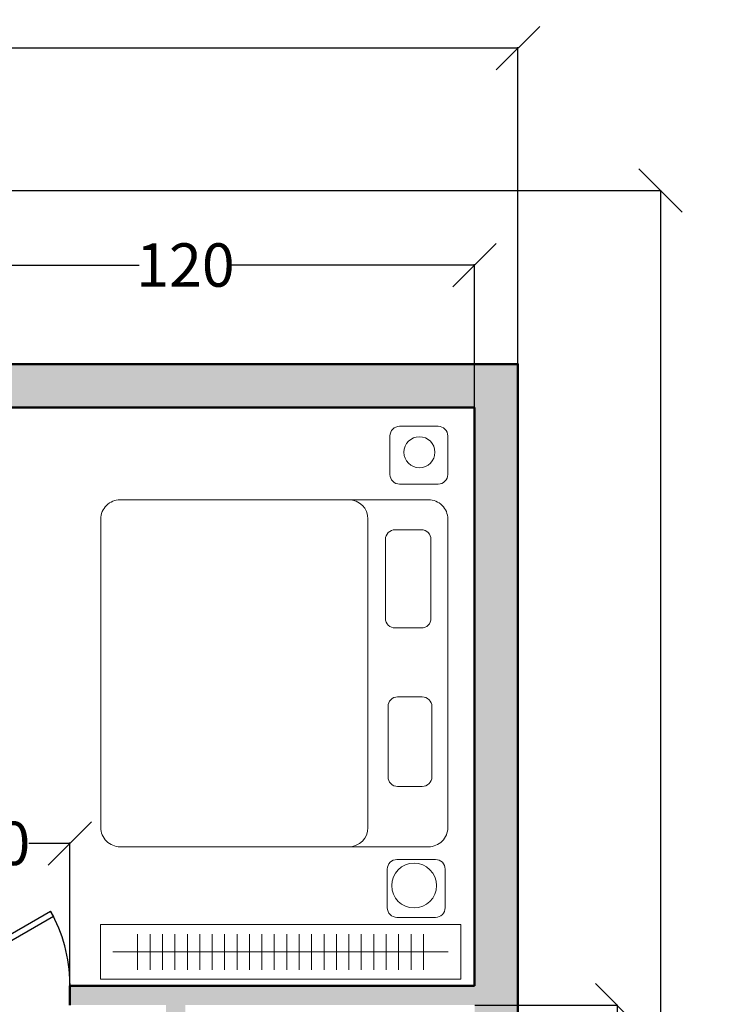
# Model space of a CAD drawing. Units: inches. Extents: x -9 to 615, y -420 to 89.
# Tile 6 of 6: x 467 to 615, y -115 to 89. Entities that reach past the tile are written whole.
import ezdxf

# ---------------------------------------------------------------- set-up
doc = ezdxf.new("R2010")
doc.units = ezdxf.units.IN
doc.header["$MEASUREMENT"] = 0
for name, color, linetype, lineweight in [('A-ANNO-DIMS', 2, 'Continuous', 18), ('A-DOOR', 4, 'Continuous', 25), ('A-FLOR-CASE', 32, 'Continuous', 18), ('A-FURN', 8, 'Continuous', 18), ('A-WALL', 7, 'Continuous', 50)]:
    doc.layers.add(name, color=color, linetype=linetype, lineweight=lineweight)
doc.layers.add('A-WALL-PATT', color=251, linetype='Continuous', lineweight=13, true_color=0x636466)
doc.styles.get("Standard").update_dxf_attribs({"font": 'arial.ttf'})
doc.dimstyles.get("Standard").update_dxf_attribs({"dimtxt": 9, "dimasz": 9, "dimexe": 0.18, "dimexo": 0.0625, "dimgap": 0.09, "dimtad": 0, "dimtih": 1, "dimtoh": 1, "dimdec": 0, "dimzin": 0, "dimdsep": 46, "dimlunit": 4, "dimtxsty": 'Standard', "dimblk": 'OBLIQUE', "dimblk2": 'OBLIQUE', "dimcen": 0.09, "dimadec": 0, "dimazin": 0, "dimtfac": 1, "dimtdec": 0, "dimtofl": 0, "dimtmove": 0, "dimatfit": 3, "dimldrblk": 'OBLIQUE', "dimfxl": 1, "dimtolj": 1, "dimtzin": 0, "dimarcsym": 0})

# ---------------------------------------------------------------- blocks, each defined once
blk = doc.blocks.new('6 BED')
for p, q in [((-33.45, 25.64), (30.55, 25.64)), ((-37.45, 21.64), (-37.45, -23.43)), ((34.55, 21.64), (34.55, -19.64))]:
    blk.add_line(p, q)
for points in [[(-42.69, 42.2), (-50.69, 42.2, 0.414214), (-52.69, 40.2), (-52.69, 32.2, 0.414214), (-50.69, 30.2), (-42.69, 30.2, 0.414214), (-40.69, 32.2), (-40.69, 40.2, 0.414214)], [(-33.45, 42.2), (30.55, 42.2, -0.414214), (34.55, 38.2), (34.55, -25.8, -0.414214), (30.55, -29.8), (-33.45, -29.8, -0.414214), (-37.45, -25.8), (-37.45, 38.2, -0.414214)], [(39.19, 41.65), (47.19, 41.65, -0.414214), (49.19, 39.65), (49.19, 31.65, -0.414214), (47.19, 29.65), (39.19, 29.65, -0.414214), (37.19, 31.65), (37.19, 39.65, -0.414214)], [(5.45, 38.89), (20.03, 38.89, -0.414214), (22.03, 36.89), (22.03, 31.79, -0.414214), (20.03, 29.79), (5.45, 29.79, -0.414214), (3.45, 31.79), (3.45, 36.89, -0.414214)], [(-29.22, 38.71), (-12.85, 38.71, -0.414214), (-10.85, 36.71), (-10.85, 31.26, -0.414214), (-12.85, 29.26), (-29.22, 29.26, -0.414214), (-31.22, 31.26), (-31.22, 36.71, -0.414214)]]:
    blk.add_lwpolyline(points, format="xyb", close=True)
for centre, start, end in [((-33.45, 21.64), 90, 180), ((30.55, 21.64), 0, 90)]:
    blk.add_arc(centre, 4, start, end)
blk = doc.blocks.new('*U12')
for p, q in [((0, 0), (0, -6)), ((40, 0), (40, -6))]:
    blk.add_line(p, q)
blk.add_lwpolyline([(0, 0), (34.64, 20), (35.52, 18.48), (0.87, -1.52)], close=True)
blk.add_arc((0, 0), 40, 0, 30)
blk = doc.blocks.new('_Oblique')
at = {"color": 0, "linetype": 'ByBlock', "lineweight": -2}
blk.add_line((-0.5, -0.5), (0.5, 0.5), dxfattribs=at)
blk = doc.blocks.new('*D40')
at = {"layer": 'A-ANNO-DIMS', "color": 0, "lineweight": -2, "transparency": 16777216}
for p, q in [((30.44, 18.08), (30.44, 83.75)), ((30.44, 83.57), (290.42, 83.57)), ((570.44, 83.57), (310.45, 83.57)), ((570.44, 18.08), (570.44, 83.75))]:
    blk.add_line(p, q, dxfattribs=at)
at = {"layer": 'Defpoints', "color": 0, "transparency": 16777216}
for p in [(570.44, 83.57), (30.44, 18.02), (570.44, 18.02)]:
    blk.add_point(p, dxfattribs=at)
at = {"layer": 'A-ANNO-DIMS', "color": 0, "lineweight": -2, "transparency": 16777216, "xscale": 9, "yscale": 9, "zscale": 9, "rotation": 180}
blk.add_blockref('_Oblique', (30.44, 83.57), dxfattribs=at)
at = {"layer": 'A-ANNO-DIMS', "color": 0, "lineweight": -2, "transparency": 16777216, "xscale": 9, "yscale": 9, "zscale": 9}
blk.add_blockref('_Oblique', (570.44, 83.57), dxfattribs=at)
at = {"layer": 'A-ANNO-DIMS', "color": 0, "transparency": 16777216, "insert": (300.44, 83.57), "char_height": 9, "attachment_point": 5}
blk.add_mtext('\\A1;540', dxfattribs=at)
blk = doc.blocks.new('*D42')
at = {"layer": 'A-ANNO-DIMS', "color": 0, "lineweight": -2, "transparency": 16777216}
for p, q in [((437.5, 54.02), (600.17, 54.02)), ((599.99, 54.02), (599.99, -160.45)), ((599.99, -384.29), (599.99, -169.82)), ((365.62, -384.29), (600.17, -384.29))]:
    blk.add_line(p, q, dxfattribs=at)
at = {"layer": 'Defpoints', "color": 0, "transparency": 16777216}
for p in [(437.44, 54.02), (599.99, 54.02), (365.56, -384.29)]:
    blk.add_point(p, dxfattribs=at)
at = {"layer": 'A-ANNO-DIMS', "color": 0, "lineweight": -2, "transparency": 16777216, "xscale": 9, "yscale": 9, "zscale": 9}
for p, rotation in [((599.99, 54.02), 90), ((599.99, -384.29), 270)]:
    blk.add_blockref('_Oblique', p, dxfattribs=dict(at, rotation=rotation))
at = {"layer": 'A-ANNO-DIMS', "color": 0, "transparency": 16777216, "insert": (599.99, -165.14), "char_height": 9, "attachment_point": 5}
blk.add_mtext('\\A1;438.3', dxfattribs=at)
blk = doc.blocks.new('*D47')
at = {"layer": 'A-ANNO-DIMS', "color": 0, "lineweight": -2, "transparency": 16777216}
for p, q in [((441.44, 9.08), (441.44, 38.75)), ((441.44, 38.57), (491.84, 38.57)), ((561.44, 38.57), (511.03, 38.57)), ((561.44, 9.08), (561.44, 38.75))]:
    blk.add_line(p, q, dxfattribs=at)
at = {"layer": 'Defpoints', "color": 0, "transparency": 16777216}
for p in [(561.44, 38.57), (441.44, 9.02), (561.44, 9.02)]:
    blk.add_point(p, dxfattribs=at)
at = {"layer": 'A-ANNO-DIMS', "color": 0, "lineweight": -2, "transparency": 16777216, "xscale": 9, "yscale": 9, "zscale": 9, "rotation": 180}
blk.add_blockref('_Oblique', (441.44, 38.57), dxfattribs=at)
at = {"layer": 'A-ANNO-DIMS', "color": 0, "lineweight": -2, "transparency": 16777216, "xscale": 9, "yscale": 9, "zscale": 9}
blk.add_blockref('_Oblique', (561.44, 38.57), dxfattribs=at)
at = {"layer": 'A-ANNO-DIMS', "color": 0, "transparency": 16777216, "insert": (501.44, 38.57), "char_height": 9, "attachment_point": 5}
blk.add_mtext('\\A1;120', dxfattribs=at)
blk = doc.blocks.new('*D58')
at = {"layer": 'A-ANNO-DIMS', "color": 0, "lineweight": -2, "transparency": 16777216}
for p, q in [((561.5, -114.98), (591.17, -114.98)), ((590.99, -114.98), (590.99, -152.3)), ((590.99, -198.98), (590.99, -161.67)), ((561.5, -198.98), (591.17, -198.98))]:
    blk.add_line(p, q, dxfattribs=at)
at = {"layer": 'Defpoints', "color": 0, "transparency": 16777216}
for p in [(561.44, -114.98), (561.44, -198.98), (590.99, -198.98)]:
    blk.add_point(p, dxfattribs=at)
at = {"layer": 'A-ANNO-DIMS', "color": 0, "lineweight": -2, "transparency": 16777216, "xscale": 9, "yscale": 9, "zscale": 9}
for p, rotation in [((590.99, -114.98), 90), ((590.99, -198.98), 270)]:
    blk.add_blockref('_Oblique', p, dxfattribs=dict(at, rotation=rotation))
at = {"layer": 'A-ANNO-DIMS', "color": 0, "transparency": 16777216, "insert": (590.99, -156.98), "char_height": 9, "attachment_point": 5}
blk.add_mtext('\\A1;84', dxfattribs=at)
blk = doc.blocks.new('*D82')
at = {"layer": 'A-ANNO-DIMS', "color": 0, "lineweight": -2, "transparency": 16777216}
for p, q in [((447.44, -110.92), (447.44, -81.25)), ((447.44, -81.43), (455.92, -81.43)), ((477.44, -81.43), (468.96, -81.43)), ((477.44, -110.92), (477.44, -81.25))]:
    blk.add_line(p, q, dxfattribs=at)
at = {"layer": 'Defpoints', "color": 0, "transparency": 16777216}
for p in [(477.44, -81.43), (447.44, -110.98), (477.44, -110.98)]:
    blk.add_point(p, dxfattribs=at)
at = {"layer": 'A-ANNO-DIMS', "color": 0, "lineweight": -2, "transparency": 16777216, "xscale": 9, "yscale": 9, "zscale": 9, "rotation": 180}
blk.add_blockref('_Oblique', (447.44, -81.43), dxfattribs=at)
at = {"layer": 'A-ANNO-DIMS', "color": 0, "lineweight": -2, "transparency": 16777216, "xscale": 9, "yscale": 9, "zscale": 9}
blk.add_blockref('_Oblique', (477.44, -81.43), dxfattribs=at)
at = {"layer": 'A-ANNO-DIMS', "color": 0, "transparency": 16777216, "insert": (462.44, -81.43), "char_height": 9, "attachment_point": 5}
blk.add_mtext('\\A1;30', dxfattribs=at)

msp = doc.modelspace()

# ---------------------------------------------------------------- hatches: boundary and pattern name
at = {"layer": 'A-WALL-PATT'}
h = msp.add_hatch(color=256, dxfattribs=at)
h.dxf.hatch_style = 1
h.paths.add_polyline_path([(570.4378, 18.0183), (437.4378, 18.0183), (437.4378, -14.9817), (437.4378, -110.9817), (385.4378, -110.9817), (385.4378, -114.9817), (385.4378, -120.9817), (389.4378, -120.9817), (389.4378, -114.9817), (437.4378, -114.9817), (447.4378, -114.9817), (447.4378, -110.9817), (441.4378, -110.9817), (441.4378, 9.0183), (561.4378, 9.0183), (561.4378, -110.9817), (477.4378, -110.9817), (477.4378, -114.9817), (497.4378, -114.9817), (497.4378, -168.9817), (501.4378, -168.9817), (501.4378, -114.9817), (561.4378, -114.9817), (561.4378, -198.9817), (531.4378, -198.9817), (501.4378, -198.9817), (501.4378, -192.9817), (497.4378, -192.9817), (497.4378, -198.9817), (477.4378, -198.9817), (477.4378, -202.9817), (561.4378, -202.9817), (561.4378, -332.9817), (441.4378, -332.9817), (441.4378, -202.9817), (447.4378, -202.9817), (447.4378, -198.9817), (437.4378, -198.9817), (431.4378, -198.9817), (431.4378, -202.9817), (437.4378, -202.9817), (437.4378, -256.9817), (389.4378, -256.9817), (389.4378, -202.9799), (407.5704, -202.9799), (407.4511, -198.9817), (389.4378, -198.9817), (385.4378, -198.9817), (385.4378, -302.9817), (389.4378, -302.9817), (389.4378, -260.9817), (437.4378, -260.9817), (437.4378, -332.9817), (389.4378, -332.9817), (389.4378, -326.9817), (385.4378, -326.9817), (385.4378, -332.9817), (352.4378, -332.9817), (352.4378, -341.9817), (570.4378, -341.9817)])

# ---------------------------------------------------------------- linework, layer by layer
at = {"layer": 'A-FLOR-CASE'}
for p, q in [((558.5553, -98.2285), (483.7857, -98.2285)), ((483.7857, -98.2285), (483.7857, -109.6291)), ((483.7857, -109.6291), (483.7857, -98.2285)), ((558.5553, -109.6291), (558.5553, -98.2285)), ((491.5205, -107.6291), (491.5205, -100.2285)), ((494.0987, -107.6291), (494.0987, -100.2285)), ((496.677, -107.6291), (496.677, -100.2285)), ((499.2553, -107.6291), (499.2553, -100.2285)), ((501.8335, -107.6291), (501.8335, -100.2285)), ((504.4118, -107.6291), (504.4118, -100.2285)), ((506.99, -107.6291), (506.99, -100.2285)), ((509.5683, -107.6291), (509.5683, -100.2285)), ((512.1466, -107.6291), (512.1466, -100.2285)), ((514.7248, -107.6291), (514.7248, -100.2285)), ((517.3031, -107.6291), (517.3031, -100.2285)), ((519.8814, -107.6291), (519.8814, -100.2285)), ((522.4596, -107.6291), (522.4596, -100.2285)), ((525.0379, -107.6291), (525.0379, -100.2285)), ((527.6161, -107.6291), (527.6161, -100.2285)), ((530.1944, -107.6291), (530.1944, -100.2285)), ((532.7727, -107.6291), (532.7727, -100.2285)), ((535.3509, -107.6291), (535.3509, -100.2285)), ((537.9292, -107.6291), (537.9292, -100.2285)), ((540.5074, -107.6291), (540.5074, -100.2285)), ((543.0857, -107.6291), (543.0857, -100.2285)), ((545.664, -107.6291), (545.664, -100.2285)), ((548.2422, -107.6291), (548.2422, -100.2285)), ((550.8205, -107.6291), (550.8205, -100.2285)), ((555.977, -103.9288), (486.364, -103.9288)), ((483.7857, -109.6291), (558.5553, -109.6291))]:
    msp.add_line(p, q, dxfattribs=at)
at = {"layer": 'A-FURN'}
for centre, radius in [((549.9898, -0.2717), 3.2166), ((548.8899, -90.1704), 4.6429)]:
    msp.add_circle(centre, radius, dxfattribs=at)
at = {"layer": 'A-WALL'}
for p, q in [((441.4378, 9.0183), (561.4378, 9.0183)), ((561.4378, 9.0183), (561.4378, -110.9817)), ((477.4378, -110.9817), (477.4378, -114.9817)), ((477.4378, -110.9817), (561.4378, -110.9817))]:
    msp.add_line(p, q, dxfattribs=at)
msp.add_lwpolyline([(437.4378, 18.0183), (570.4378, 18.0183), (570.4378, -341.9817), (352.4378, -341.9817)], dxfattribs=at)

# ---------------------------------------------------------------- block references
at = {"layer": 'A-DOOR', "xscale": 0.75, "yscale": 0.75, "zscale": 0.75}
msp.add_blockref('*U12', (447.4378, -110.4817), dxfattribs=at)
at = {"layer": 'A-FURN', "rotation": 270}
msp.add_blockref('6 BED', (513.6781, -47.5804), dxfattribs=at)

# ---------------------------------------------------------------- dimensions: what is measured, and where the dimension line sits
at = {"layer": 'A-ANNO-DIMS'}
for base, p1, p2, picture, middle in [((570.4378, 83.5683), (30.4378, 18.0183), (570.4378, 18.0183), '*D40', (300.4378, 83.5683)), ((561.4378, 38.5683), (441.4378, 9.0183), (561.4378, 9.0183), '*D47', (501.4378, 38.5683)), ((477.4378, -81.4317), (447.4378, -110.9817), (477.4378, -110.9817), '*D82', (462.4378, -81.4317))]:
    dim = msp.add_linear_dim(base=base, p1=p1, p2=p2, dimstyle='Standard', override={"dimdec": 0, "dimlfac": 1, "dimrnd": 0, "dimzin": 0, "dimdsep": 46, "dimlunit": 2}, dxfattribs=at)
    dim.commit()
    dim.dimension.update_dxf_attribs({"geometry": picture, "text_midpoint": middle})
for base, p1, p2, angle, override, picture, middle in [((599.9878, 54.0183), (365.5581, -384.2897), (437.4378, 54.0183), 90, {"dimdec": 1, "dimlfac": 1, "dimrnd": 0, "dimzin": 0, "dimdsep": 46, "dimlunit": 2}, '*D42', (599.9878, -165.1357)), ((590.9878, -198.9817), (561.4378, -114.9817), (561.4378, -198.9817), 270, {"dimdec": 0, "dimlfac": 1, "dimrnd": 0, "dimzin": 0, "dimdsep": 46, "dimlunit": 2}, '*D58', (590.9878, -156.9817))]:
    dim = msp.add_linear_dim(base=base, p1=p1, p2=p2, angle=angle, dimstyle='Standard', override=override, dxfattribs=at)
    dim.commit()
    dim.dimension.update_dxf_attribs({"geometry": picture, "text_midpoint": middle})

doc.saveas('drawing.dxf')
